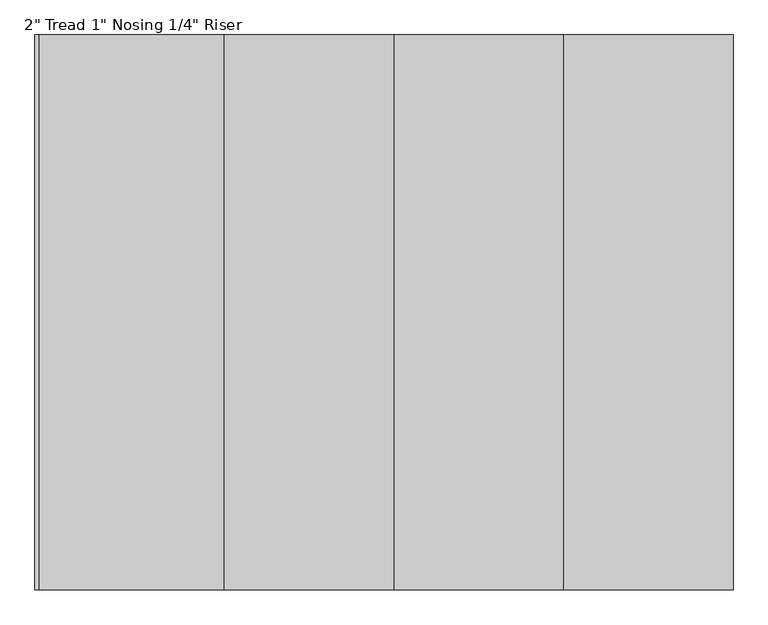
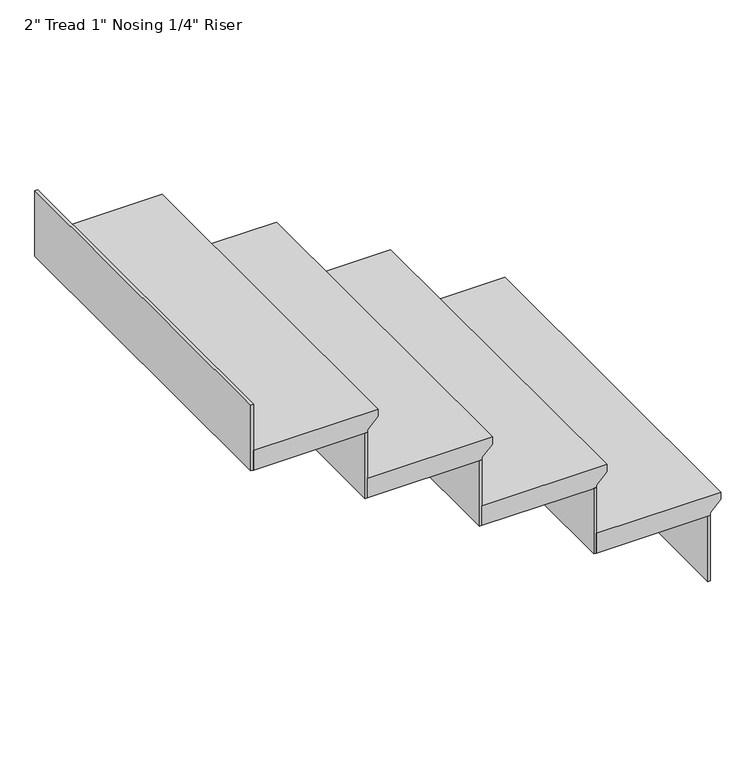
"""IFC4 building model written with IfcOpenShell, lengths in millimetres: stair flight geometry."""

from ifc_helpers import new_model, si_unit, frame, origin, place, context, project, spatial, polyline, outline, extrude, source, transform, mapped, element, save


def stair_flight_82b2d532(model_context):
    return source(origin(), model_context, "Body", "SweptSolid", [
        extrude(outline(polyline([(2370.6666667, -803.1608498), (2370.6666667, -1107.9608498), (2319.8666667, -1107.9608498), (2319.8666667, -828.5608498), (2326.2166667, -828.5608498), (2351.6166667, -803.1608498), (2370.6666667, -803.1608498)])), frame((0.0, 1203.1115866, 0.0), z_axis=(0.0, 1.0, 0.0), x_axis=(0.0, 0.0, 1.0)), (0.0, 0.0, 1.0), 914.4),
        extrude(outline(polyline([(-834.9108498, 2117.5115866), (-828.5608498, 2117.5115866), (-828.5608498, 1203.1115866), (-834.9108498, 1203.1115866), (-834.9108498, 2117.5115866)])), frame((0.0, 0.0, 2150.5333333), z_axis=(0.0, 0.0, 1.0), x_axis=(1.0, 0.0, 0.0)), (0.0, 0.0, 1.0), 169.3333333),
        extrude(outline(polyline([(-1114.3108498, 2117.5115866), (-1107.9608498, 2117.5115866), (-1107.9608498, 1203.1115866), (-1114.3108498, 1203.1115866), (-1114.3108498, 2117.5115866)])), frame((0.0, 0.0, 2319.8666667), z_axis=(0.0, 0.0, 1.0), x_axis=(1.0, 0.0, 0.0)), (0.0, 0.0, 1.0), 169.3333333),
        extrude(outline(polyline([(2540.0, -1082.5608498), (2540.0, -1387.3608498), (2489.2, -1387.3608498), (2489.2, -1107.9608498), (2495.55, -1107.9608498), (2520.95, -1082.5608498), (2540.0, -1082.5608498)])), frame((0.0, 1203.1115866, 0.0), z_axis=(0.0, 1.0, 0.0), x_axis=(0.0, 0.0, 1.0)), (0.0, 0.0, 1.0), 914.4),
        extrude(outline(polyline([(-1393.7108498, 2117.5115866), (-1387.3608498, 2117.5115866), (-1387.3608498, 1203.1115866), (-1393.7108498, 1203.1115866), (-1393.7108498, 2117.5115866)])), frame((0.0, 0.0, 2489.2), z_axis=(0.0, 0.0, 1.0), x_axis=(1.0, 0.0, 0.0)), (0.0, 0.0, 1.0), 169.3333333),
        extrude(outline(polyline([(2709.3333333, -1361.9608498), (2709.3333333, -1666.7608498), (2658.5333333, -1666.7608498), (2658.5333333, -1387.3608498), (2664.8833333, -1387.3608498), (2690.2833333, -1361.9608498), (2709.3333333, -1361.9608498)])), frame((0.0, 1203.1115866, 0.0), z_axis=(0.0, 1.0, 0.0), x_axis=(0.0, 0.0, 1.0)), (0.0, 0.0, 1.0), 914.4),
        extrude(outline(polyline([(-1673.1108498, 2117.5115866), (-1666.7608498, 2117.5115866), (-1666.7608498, 1203.1115866), (-1673.1108498, 1203.1115866), (-1673.1108498, 2117.5115866)])), frame((0.0, 0.0, 2658.5333333), z_axis=(0.0, 0.0, 1.0), x_axis=(1.0, 0.0, 0.0)), (0.0, 0.0, 1.0), 169.3333333),
        extrude(outline(polyline([(-1952.5108498, 2117.5115866), (-1946.1608498, 2117.5115866), (-1946.1608498, 1203.1115866), (-1952.5108498, 1203.1115866), (-1952.5108498, 2117.5115866)])), frame((0.0, 0.0, 2827.8666667), z_axis=(0.0, 0.0, 1.0), x_axis=(1.0, 0.0, 0.0)), (0.0, 0.0, 1.0), 169.3333333),
        extrude(outline(polyline([(2878.6666667, -1641.3608498), (2878.6666667, -1946.1608498), (2827.8666667, -1946.1608498), (2827.8666667, -1666.7608498), (2834.2166667, -1666.7608498), (2859.6166667, -1641.3608498), (2878.6666667, -1641.3608498)])), frame((0.0, 1203.1115866, 0.0), z_axis=(0.0, 1.0, 0.0), x_axis=(0.0, 0.0, 1.0)), (0.0, 0.0, 1.0), 914.4),
    ])


if __name__ == "__main__":
    model = new_model("IFC4")
    model_context = context("Model", 3, world=origin())
    ifc_project = project(units=[si_unit("LENGTHUNIT", "METRE", prefix="MILLI")], contexts=[model_context])
    site = spatial("IfcSite", under=ifc_project)
    building = spatial("IfcBuilding", under=site)
    placement = place(None, origin())
    stair_flight_shape = stair_flight_82b2d532(model_context)
    element("IfcStairFlight", 1, ObjectType="2\" Tread 1\" Nosing 1/4\" Riser", at=placement, inside=building, context=model_context, shape_type="MappedRepresentation", body=[
        mapped(stair_flight_shape, transform((0.0, 0.0, 0.0), x_axis=(1.0, 0.0, 0.0), y_axis=(0.0, 1.0, 0.0), z_axis=(0.0, 0.0, 1.0))),
    ])
    save(model, "model.ifc")
